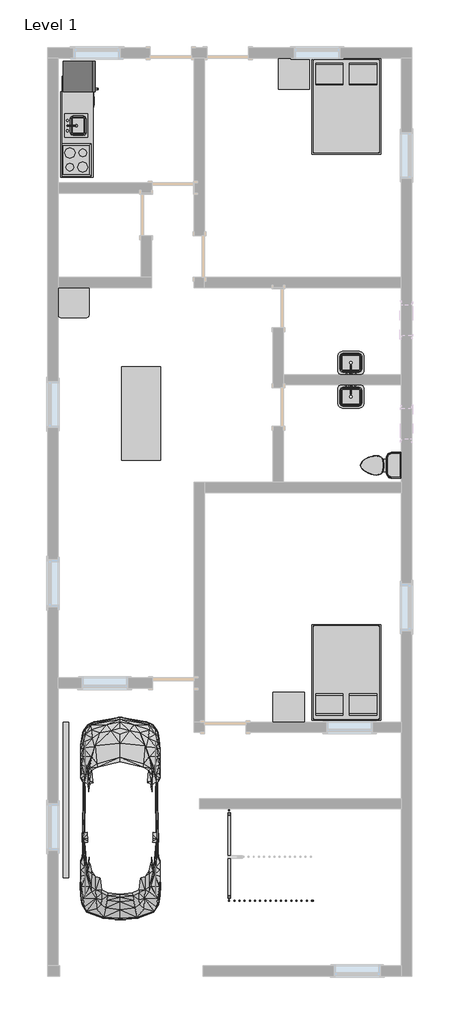
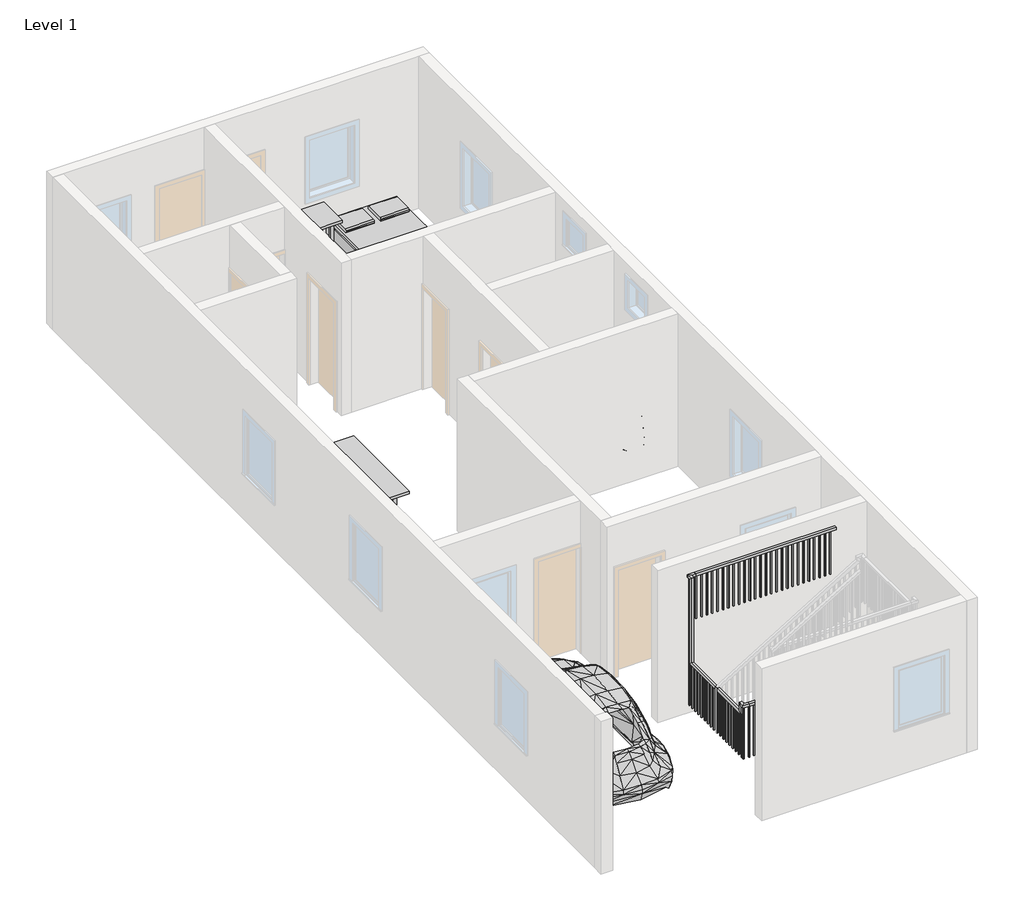
# One storey, part 3 of 3: 7 furniture elements, 6 proxies, 4 flow terminals, 1 railing.
"""IFC4 building model written with IfcOpenShell, lengths in millimetres."""

from ifc_helpers import new_model, si_unit, frame, origin, place, context, project, spatial, polyline, outline, extrude, faceted_brep, transform, mapped, element, save
from components import proxy_a6faaae8, proxy_45b28599, kitchenette_medium_kitchenette_medium_844211aa, parking_space_9_x_18_90_deg_2dcab977, rpc_beetle_rpc_beetle_3ce7ba48, proxy_c523a7b7, flow_terminal_871c2e40, flow_terminal_62a433f7, toilet_domestic_3d_toilet_domestic_3d_f7549cf7, toilet_domestic_3d_toilet_domestic_3d_183bbd19, furniture_c8abb964, furniture_1781b5df, furniture_bcf351fa, furniture_5bc9ed15, furniture_a5b052b6

model = new_model("IFC4")

# Units and contexts
model_context = context("Model", 3, world=origin())
ifc_project = project(units=[si_unit("LENGTHUNIT", "METRE", prefix="MILLI")], contexts=[model_context])

# Site, building, storey
site = spatial("IfcSite", under=ifc_project)
building = spatial("IfcBuilding", under=site)
storey = spatial("IfcBuildingStorey", under=building, Name="Level 1", Elevation=0.0)

# Proxies
placement = place(None, origin())
proxy_shape = proxy_a6faaae8(model_context)
element("IfcBuildingElementProxy", 1, Name="Cook Top-4 Unit2 : 22\" x 20\"", ObjectType="Cook Top-4 Unit2 : 22\" x 20\"", at=placement, inside=storey, context=model_context, shape_type="MappedRepresentation", body=[
    mapped(proxy_shape, transform((-9361.8283387, 8629.5865244, 0.0), x_axis=(0.0, 1.0, 0.0), y_axis=(-1.0, 0.0, 0.0), z_axis=(0.0, 0.0, 1.0))),
])
proxy_2_shape = proxy_45b28599(model_context)
element("IfcBuildingElementProxy", 2, Name="Dishwasher : 24\" x 24\" x 34\"", ObjectType="Dishwasher : 24\" x 24\" x 34\"", at=placement, inside=storey, context=model_context, shape_type="MappedRepresentation", body=[
    mapped(proxy_2_shape, transform((-9069.978774, 9580.7690559, 0.0), x_axis=(0.0, 1.0, 0.0), y_axis=(-1.0, 0.0, 0.0), z_axis=(0.0, 0.0, 1.0))),
])
kitchenette_medium_kitchenette_medium_shape = kitchenette_medium_kitchenette_medium_844211aa(model_context)
element("IfcBuildingElementProxy", 3, Name="Kitchenette - Medium : Kitchenette - Medium", ObjectType="Kitchenette - Medium : Kitchenette - Medium", at=placement, inside=storey, context=model_context, shape_type="MappedRepresentation", body=[
    mapped(kitchenette_medium_kitchenette_medium_shape, transform((-9666.6283387, 8953.7488195, 0.0), x_axis=(0.0, 1.0, 0.0), y_axis=(-1.0, 0.0, 0.0), z_axis=(0.0, 0.0, 1.0))),
])
parking_space_9_x_18_90_deg_shape = parking_space_9_x_18_90_deg_2dcab977(model_context)
element("IfcBuildingElementProxy", 4, Name="Parking Space : 9' x 18' - 90 deg", ObjectType="Parking Space : 9' x 18' - 90 deg", at=placement, inside=storey, context=model_context, shape_type="MappedRepresentation", body=[
    mapped(parking_space_9_x_18_90_deg_shape, transform((-9564.1370113, -2381.3134756, 0.0), x_axis=(1.0, 0.0, 0.0), y_axis=(0.0, 1.0, 0.0), z_axis=(0.0, 0.0, 1.0))),
])
rpc_beetle_rpc_beetle_shape = rpc_beetle_rpc_beetle_3ce7ba48(model_context)
element("IfcBuildingElementProxy", 5, Name="RPC Beetle : RPC Beetle", ObjectType="RPC Beetle : RPC Beetle", at=placement, inside=storey, context=model_context, shape_type="MappedRepresentation", body=[
    mapped(rpc_beetle_rpc_beetle_shape, transform((-8497.3370113, -5505.5134756, 0.0), x_axis=(1.0, 0.0, 0.0), y_axis=(0.0, 1.0, 0.0), z_axis=(0.0, 0.0, 1.0))),
])
proxy_3_shape = proxy_c523a7b7(model_context)
element("IfcBuildingElementProxy", 6, Name="Refrigerator : 24\" x 25\" LH", ObjectType="Refrigerator : 24\" x 25\" LH", at=placement, inside=storey, context=model_context, shape_type="MappedRepresentation", body=[
    mapped(proxy_3_shape, transform((-9316.1793673, 10261.5365244, 0.0), x_axis=(0.0, 1.0, 0.0), y_axis=(-1.0, 0.0, 0.0), z_axis=(0.0, 0.0, 1.0))),
])

# Flow terminals
flow_terminal_shape = flow_terminal_871c2e40(model_context)
element("IfcFlowTerminal", 7, ObjectType="Sink Kitchen-Island : 18\" x 18\"", at=placement, inside=storey, context=model_context, shape_type="MappedRepresentation", body=[
    mapped(flow_terminal_shape, transform((-9359.4829376, 9286.9972838, -14.4), x_axis=(0.0, 1.0, 0.0), y_axis=(-1.0, 0.0, 0.0), z_axis=(0.0, 0.0, 1.0))),
])
flow_terminal_2_shape = flow_terminal_62a433f7(model_context)
element("IfcFlowTerminal", 8, ObjectType="Sink Vanity-Square : 20\" x 18\"", at=placement, inside=storey, context=model_context, shape_type="MappedRepresentation", body=[
    mapped(flow_terminal_2_shape, transform((-3960.4477707, 4606.0319255, 0.0), x_axis=(-1.0000000000000004, 0.0, 0.0), y_axis=(0.0, -1.0000000000000004, 0.0), z_axis=(0.0, 0.0, 1.0))),
])
element("IfcFlowTerminal", 9, ObjectType="Sink Vanity-Square : 20\" x 18\"", at=placement, inside=storey, context=model_context, shape_type="MappedRepresentation", body=[
    mapped(flow_terminal_2_shape, transform((-3991.8262519, 4042.5411233, 0.0), x_axis=(1.0, 0.0, 0.0), y_axis=(0.0, 1.0, 0.0), z_axis=(0.0, 0.0, 1.0))),
])
toilet_domestic_3d_toilet_domestic_3d_shape = toilet_domestic_3d_toilet_domestic_3d_f7549cf7(model_context)
toilet_domestic_3d_toilet_domestic_3d_2_shape = toilet_domestic_3d_toilet_domestic_3d_183bbd19(model_context)
element("IfcFlowTerminal", 10, ObjectType="Toilet-Domestic-3D : Toilet-Domestic-3D", at=placement, inside=storey, context=model_context, shape_type="MappedRepresentation", body=[
    mapped(toilet_domestic_3d_toilet_domestic_3d_shape, transform((-3480.2330387, 2647.8865244, 0.0), x_axis=(0.0, -1.0000000000000004, 0.0), y_axis=(1.0000000000000004, 0.0, 0.0), z_axis=(0.0, 0.0, 1.0))),
    mapped(toilet_domestic_3d_toilet_domestic_3d_2_shape, transform((-3480.2330387, 2647.8865244, 0.0), x_axis=(0.0, -1.0000000000000004, 0.0), y_axis=(1.0000000000000004, 0.0, 0.0), z_axis=(0.0, 0.0, 1.0))),
])

# Furniture
furniture_shape = furniture_c8abb964(model_context)
element("IfcFurniture", 11, ObjectType="Bed-Box : Double 53\" x 74\"", at=placement, inside=storey, context=model_context, shape_type="MappedRepresentation", body=[
    mapped(furniture_shape, transform((-4404.1894703, 9918.1160326, 0.0), x_axis=(1.0, 0.0, 0.0), y_axis=(0.0, 1.0, 0.0), z_axis=(0.0, 0.0, 1.0))),
])
element("IfcFurniture", 12, ObjectType="Bed-Box : Double 53\" x 74\"", at=placement, inside=storey, context=model_context, shape_type="MappedRepresentation", body=[
    mapped(furniture_shape, transform((-3725.8845523, -1644.7134756, 0.0), x_axis=(-1.0000000000000004, 0.0, 0.0), y_axis=(0.0, -1.0000000000000004, 0.0), z_axis=(0.0, 0.0, 1.0))),
])
furniture_2_shape = furniture_1781b5df(model_context)
element("IfcFurniture", 13, ObjectType="Counter Top w Sink Hole : 24\" Depth", at=placement, inside=storey, context=model_context, shape_type="MappedRepresentation", body=[
    mapped(furniture_2_shape, transform((-9666.6283387, 9487.1488195, -14.4), x_axis=(0.0, 1.0, 0.0), y_axis=(-1.0, 0.0, 0.0), z_axis=(0.0, 0.0, 1.0))),
])
furniture_3_shape = furniture_bcf351fa(model_context)
element("IfcFurniture", 14, ObjectType="Table-End : 24\" x 24\"", at=placement, inside=storey, context=model_context, shape_type="MappedRepresentation", body=[
    mapped(furniture_3_shape, transform((-9720.2706416, 5695.8865244, 0.0), x_axis=(1.0, 0.0, 0.0), y_axis=(0.0, 1.0, 0.0), z_axis=(0.0, 0.0, 1.0))),
])
furniture_4_shape = furniture_5bc9ed15(model_context)
element("IfcFurniture", 15, ObjectType="Table-Night Stand : 24\" x 24\" x 30\"", at=placement, inside=storey, context=model_context, shape_type="MappedRepresentation", body=[
    mapped(furniture_4_shape, transform((-5503.8706416, -2406.7134756, 0.0), x_axis=(1.0, 0.0, 0.0), y_axis=(0.0, 1.0, 0.0), z_axis=(0.0, 0.0, 1.0))),
])
element("IfcFurniture", 16, ObjectType="Table-Night Stand : 24\" x 24\" x 30\"", at=placement, inside=storey, context=model_context, shape_type="MappedRepresentation", body=[
    mapped(furniture_4_shape, transform((-5402.2706416, 10013.8865244, 0.0), x_axis=(1.0, 0.0, 0.0), y_axis=(0.0, 1.0, 0.0), z_axis=(0.0, 0.0, 1.0))),
])
furniture_5_shape = furniture_a5b052b6(model_context)
element("IfcFurniture", 17, ObjectType="Table-Rectangular : 72\" x 30\"", at=placement, inside=storey, context=model_context, shape_type="MappedRepresentation", body=[
    mapped(furniture_5_shape, transform((-8090.9370113, 3663.8865244, 0.0), x_axis=(0.0, 1.0, 0.0), y_axis=(-1.0, 0.0, 0.0), z_axis=(0.0, 0.0, 1.0))),
])

# Railing
element("IfcRailing", 18, ObjectType="Handrail - Rectangular", at=placement, inside=storey, context=model_context, shape_type="SolidModel", body=[
    faceted_brep([(-4712.7370113, -5909.6215145, 1253.0666667), (-4712.7370113, -5909.6215145, 1202.2666667), (-4712.7370113, -5858.8215145, 1202.2666667), (-4712.7370113, -5858.8215145, 1253.0666667), (-6262.1370113, -5909.6215145, 1253.0666667), (-6262.1370113, -5909.6215145, 1202.2666667), (-6262.1370113, -5858.8215145, 1202.2666667), (-6262.1370113, -5858.8215145, 1253.0666667), (-6389.1370113, -5909.6215145, 1253.0666667), (-6389.1370113, -5909.6215145, 1202.2666667), (-6338.3370113, -5858.8215145, 1202.2666667), (-6338.3370113, -5858.8215145, 1253.0666667), (-6389.1370113, -5782.6215145, 1253.0666667), (-6389.1370113, -5833.4215145, 1202.2666667), (-6338.3370113, -5833.4215145, 1202.2666667), (-6338.3370113, -5782.6215145, 1253.0666667), (-6389.1370113, -5782.6215145, 1083.7333333), (-6389.1370113, -5833.4215145, 1032.9333333), (-6338.3370113, -5833.4215145, 1032.9333333), (-6338.3370113, -5782.6215145, 1083.7333333), (-6389.1370113, -4211.9518521, 1083.7333333), (-6389.1370113, -4161.1518521, 1032.9333333), (-6338.3370113, -4161.1518521, 1032.9333333), (-6338.3370113, -4211.9518521, 1083.7333333), (-6389.1370113, -4211.9518521, 2777.0666667), (-6389.1370113, -4161.1518521, 2726.2666667), (-6338.3370113, -4161.1518521, 2726.2666667), (-6338.3370113, -4211.9518521, 2777.0666667), (-6389.1370113, -4084.9518521, 2777.0666667), (-6389.1370113, -4084.9518521, 2726.2666667), (-6338.3370113, -4135.7518521, 2726.2666667), (-6338.3370113, -4135.7518521, 2777.0666667), (-6262.1370113, -4084.9518521, 2777.0666667), (-6262.1370113, -4084.9518521, 2726.2666667), (-6262.1370113, -4135.7518521, 2726.2666667), (-6262.1370113, -4135.7518521, 2777.0666667), (-3595.1370113, -4084.9518521, 2777.0666667), (-3595.1370113, -4135.7518521, 2777.0666667), (-3595.1370113, -4135.7518521, 2726.2666667), (-3595.1370113, -4084.9518521, 2726.2666667)], [[[0, 1, 2, 3]], [[1, 0, 4, 5]], [[2, 1, 5, 6]], [[3, 2, 6, 7]], [[0, 3, 7, 4]], [[5, 4, 8, 9]], [[6, 5, 9, 10]], [[7, 6, 10, 11]], [[4, 7, 11, 8]], [[9, 8, 12, 13]], [[10, 9, 13, 14]], [[11, 10, 14, 15]], [[8, 11, 15, 12]], [[13, 12, 16, 17]], [[14, 13, 17, 18]], [[15, 14, 18, 19]], [[12, 15, 19, 16]], [[17, 16, 20, 21]], [[18, 17, 21, 22]], [[19, 18, 22, 23]], [[16, 19, 23, 20]], [[21, 20, 24, 25]], [[22, 21, 25, 26]], [[23, 22, 26, 27]], [[20, 23, 27, 24]], [[25, 24, 28, 29]], [[26, 25, 29, 30]], [[27, 26, 30, 31]], [[24, 27, 31, 28]], [[29, 28, 32, 33]], [[30, 29, 33, 34]], [[31, 30, 34, 35]], [[28, 31, 35, 32]], [[36, 37, 38, 39]], [[33, 32, 36, 39]], [[34, 33, 39, 38]], [[35, 34, 38, 37]], [[32, 35, 37, 36]]]),
    faceted_brep([(-3595.1370113, -4084.9518521, 2777.0666667), (-3595.1370113, -4084.9518521, 2726.2666667), (-3595.1370113, -4034.1518521, 2726.2666667), (-3595.1370113, -4034.1518521, 2777.0666667), (-6389.1370113, -4084.9518521, 2777.0666667), (-6389.1370113, -4034.1518521, 2777.0666667), (-6389.1370113, -4034.1518521, 2726.2666667), (-6389.1370113, -4084.9518521, 2726.2666667)], [[[0, 1, 2, 3]], [[4, 5, 6, 7]], [[1, 0, 4, 7]], [[2, 1, 7, 6]], [[3, 2, 6, 5]], [[0, 3, 5, 4]]]),
    extrude(outline(polyline([(-4747.6620113, -5893.7465145), (-4747.6620113, -5874.6965145), (-4728.6120113, -5874.6965145), (-4728.6120113, -5893.7465145), (-4747.6620113, -5893.7465145)])), frame((0.0, 0.0, 169.3333333), z_axis=(0.0, 0.0, 1.0), x_axis=(1.0, 0.0, 0.0)), (0.0, 0.0, 1.0), 1032.9333333),
    extrude(outline(polyline([(-4849.2620113, -5893.7465145), (-4849.2620113, -5874.6965145), (-4830.2120113, -5874.6965145), (-4830.2120113, -5893.7465145), (-4849.2620113, -5893.7465145)])), frame((0.0, 0.0, 169.3333333), z_axis=(0.0, 0.0, 1.0), x_axis=(1.0, 0.0, 0.0)), (0.0, 0.0, 1.0), 1032.9333333),
    extrude(outline(polyline([(-4950.8620113, -5893.7465145), (-4950.8620113, -5874.6965145), (-4931.8120113, -5874.6965145), (-4931.8120113, -5893.7465145), (-4950.8620113, -5893.7465145)])), frame((0.0, 0.0, 169.3333333), z_axis=(0.0, 0.0, 1.0), x_axis=(1.0, 0.0, 0.0)), (0.0, 0.0, 1.0), 1032.9333333),
    extrude(outline(polyline([(-5052.4620113, -5893.7465145), (-5052.4620113, -5874.6965145), (-5033.4120113, -5874.6965145), (-5033.4120113, -5893.7465145), (-5052.4620113, -5893.7465145)])), frame((0.0, 0.0, 169.3333333), z_axis=(0.0, 0.0, 1.0), x_axis=(1.0, 0.0, 0.0)), (0.0, 0.0, 1.0), 1032.9333333),
    extrude(outline(polyline([(-5154.0620113, -5893.7465145), (-5154.0620113, -5874.6965145), (-5135.0120113, -5874.6965145), (-5135.0120113, -5893.7465145), (-5154.0620113, -5893.7465145)])), frame((0.0, 0.0, 169.3333333), z_axis=(0.0, 0.0, 1.0), x_axis=(1.0, 0.0, 0.0)), (0.0, 0.0, 1.0), 1032.9333333),
    extrude(outline(polyline([(-5255.6620113, -5893.7465145), (-5255.6620113, -5874.6965145), (-5236.6120113, -5874.6965145), (-5236.6120113, -5893.7465145), (-5255.6620113, -5893.7465145)])), frame((0.0, 0.0, 169.3333333), z_axis=(0.0, 0.0, 1.0), x_axis=(1.0, 0.0, 0.0)), (0.0, 0.0, 1.0), 1032.9333333),
    extrude(outline(polyline([(-5357.2620113, -5893.7465145), (-5357.2620113, -5874.6965145), (-5338.2120113, -5874.6965145), (-5338.2120113, -5893.7465145), (-5357.2620113, -5893.7465145)])), frame((0.0, 0.0, 169.3333333), z_axis=(0.0, 0.0, 1.0), x_axis=(1.0, 0.0, 0.0)), (0.0, 0.0, 1.0), 1032.9333333),
    extrude(outline(polyline([(-5458.8620113, -5893.7465145), (-5458.8620113, -5874.6965145), (-5439.8120113, -5874.6965145), (-5439.8120113, -5893.7465145), (-5458.8620113, -5893.7465145)])), frame((0.0, 0.0, 169.3333333), z_axis=(0.0, 0.0, 1.0), x_axis=(1.0, 0.0, 0.0)), (0.0, 0.0, 1.0), 1032.9333333),
    extrude(outline(polyline([(-5560.4620113, -5893.7465145), (-5560.4620113, -5874.6965145), (-5541.4120113, -5874.6965145), (-5541.4120113, -5893.7465145), (-5560.4620113, -5893.7465145)])), frame((0.0, 0.0, 169.3333333), z_axis=(0.0, 0.0, 1.0), x_axis=(1.0, 0.0, 0.0)), (0.0, 0.0, 1.0), 1032.9333333),
    extrude(outline(polyline([(-5662.0620113, -5893.7465145), (-5662.0620113, -5874.6965145), (-5643.0120113, -5874.6965145), (-5643.0120113, -5893.7465145), (-5662.0620113, -5893.7465145)])), frame((0.0, 0.0, 169.3333333), z_axis=(0.0, 0.0, 1.0), x_axis=(1.0, 0.0, 0.0)), (0.0, 0.0, 1.0), 1032.9333333),
    extrude(outline(polyline([(-5763.6620113, -5893.7465145), (-5763.6620113, -5874.6965145), (-5744.6120113, -5874.6965145), (-5744.6120113, -5893.7465145), (-5763.6620113, -5893.7465145)])), frame((0.0, 0.0, 169.3333333), z_axis=(0.0, 0.0, 1.0), x_axis=(1.0, 0.0, 0.0)), (0.0, 0.0, 1.0), 1032.9333333),
    extrude(outline(polyline([(-5865.2620113, -5893.7465145), (-5865.2620113, -5874.6965145), (-5846.2120113, -5874.6965145), (-5846.2120113, -5893.7465145), (-5865.2620113, -5893.7465145)])), frame((0.0, 0.0, 169.3333333), z_axis=(0.0, 0.0, 1.0), x_axis=(1.0, 0.0, 0.0)), (0.0, 0.0, 1.0), 1032.9333333),
    extrude(outline(polyline([(-5966.8620113, -5893.7465145), (-5966.8620113, -5874.6965145), (-5947.8120113, -5874.6965145), (-5947.8120113, -5893.7465145), (-5966.8620113, -5893.7465145)])), frame((0.0, 0.0, 169.3333333), z_axis=(0.0, 0.0, 1.0), x_axis=(1.0, 0.0, 0.0)), (0.0, 0.0, 1.0), 1032.9333333),
    extrude(outline(polyline([(-6068.4620113, -5893.7465145), (-6068.4620113, -5874.6965145), (-6049.4120113, -5874.6965145), (-6049.4120113, -5893.7465145), (-6068.4620113, -5893.7465145)])), frame((0.0, 0.0, 169.3333333), z_axis=(0.0, 0.0, 1.0), x_axis=(1.0, 0.0, 0.0)), (0.0, 0.0, 1.0), 1032.9333333),
    extrude(outline(polyline([(-6170.0620113, -5893.7465145), (-6170.0620113, -5874.6965145), (-6151.0120113, -5874.6965145), (-6151.0120113, -5893.7465145), (-6170.0620113, -5893.7465145)])), frame((0.0, 0.0, 169.3333333), z_axis=(0.0, 0.0, 1.0), x_axis=(1.0, 0.0, 0.0)), (0.0, 0.0, 1.0), 1032.9333333),
    extrude(outline(polyline([(-6271.6620113, -5893.7465145), (-6271.6620113, -5874.6965145), (-6252.6120113, -5874.6965145), (-6252.6120113, -5893.7465145), (-6271.6620113, -5893.7465145)])), frame((0.0, 0.0, 169.3333333), z_axis=(0.0, 0.0, 1.0), x_axis=(1.0, 0.0, 0.0)), (0.0, 0.0, 1.0), 1032.9333333),
    extrude(outline(polyline([(-6373.2620113, -5828.0268521), (-6354.2120113, -5828.0268521), (-6354.2120113, -5847.0768521), (-6373.2620113, -5847.0768521), (-6373.2620113, -5828.0268521)])), frame((0.0, 0.0, 169.3333333), z_axis=(0.0, 0.0, 1.0), x_axis=(1.0, 0.0, 0.0)), (0.0, 0.0, 1.0), 863.6),
    extrude(outline(polyline([(-6373.2620113, -5726.4268521), (-6354.2120113, -5726.4268521), (-6354.2120113, -5745.4768521), (-6373.2620113, -5745.4768521), (-6373.2620113, -5726.4268521)])), frame((0.0, 0.0, 169.3333333), z_axis=(0.0, 0.0, 1.0), x_axis=(1.0, 0.0, 0.0)), (0.0, 0.0, 1.0), 863.6),
    extrude(outline(polyline([(-6373.2620113, -5624.8268521), (-6354.2120113, -5624.8268521), (-6354.2120113, -5643.8768521), (-6373.2620113, -5643.8768521), (-6373.2620113, -5624.8268521)])), frame((0.0, 0.0, 169.3333333), z_axis=(0.0, 0.0, 1.0), x_axis=(1.0, 0.0, 0.0)), (0.0, 0.0, 1.0), 863.6),
    extrude(outline(polyline([(-6373.2620113, -5523.2268521), (-6354.2120113, -5523.2268521), (-6354.2120113, -5542.2768521), (-6373.2620113, -5542.2768521), (-6373.2620113, -5523.2268521)])), frame((0.0, 0.0, 169.3333333), z_axis=(0.0, 0.0, 1.0), x_axis=(1.0, 0.0, 0.0)), (0.0, 0.0, 1.0), 863.6),
    extrude(outline(polyline([(-6373.2620113, -5421.6268521), (-6354.2120113, -5421.6268521), (-6354.2120113, -5440.6768521), (-6373.2620113, -5440.6768521), (-6373.2620113, -5421.6268521)])), frame((0.0, 0.0, 169.3333333), z_axis=(0.0, 0.0, 1.0), x_axis=(1.0, 0.0, 0.0)), (0.0, 0.0, 1.0), 863.6),
    extrude(outline(polyline([(-6373.2620113, -5320.0268521), (-6354.2120113, -5320.0268521), (-6354.2120113, -5339.0768521), (-6373.2620113, -5339.0768521), (-6373.2620113, -5320.0268521)])), frame((0.0, 0.0, 169.3333333), z_axis=(0.0, 0.0, 1.0), x_axis=(1.0, 0.0, 0.0)), (0.0, 0.0, 1.0), 863.6),
    extrude(outline(polyline([(-6373.2620113, -5218.4268521), (-6354.2120113, -5218.4268521), (-6354.2120113, -5237.4768521), (-6373.2620113, -5237.4768521), (-6373.2620113, -5218.4268521)])), frame((0.0, 0.0, 169.3333333), z_axis=(0.0, 0.0, 1.0), x_axis=(1.0, 0.0, 0.0)), (0.0, 0.0, 1.0), 863.6),
    extrude(outline(polyline([(-6373.2620113, -5116.8268521), (-6354.2120113, -5116.8268521), (-6354.2120113, -5135.8768521), (-6373.2620113, -5135.8768521), (-6373.2620113, -5116.8268521)])), frame((0.0, 0.0, 169.3333333), z_axis=(0.0, 0.0, 1.0), x_axis=(1.0, 0.0, 0.0)), (0.0, 0.0, 1.0), 863.6),
    extrude(outline(polyline([(-6373.2620113, -5015.2268521), (-6354.2120113, -5015.2268521), (-6354.2120113, -5034.2768521), (-6373.2620113, -5034.2768521), (-6373.2620113, -5015.2268521)])), frame((0.0, 0.0, 169.3333333), z_axis=(0.0, 0.0, 1.0), x_axis=(1.0, 0.0, 0.0)), (0.0, 0.0, 1.0), 863.6),
    extrude(outline(polyline([(-6373.2620113, -4913.6268521), (-6354.2120113, -4913.6268521), (-6354.2120113, -4932.6768521), (-6373.2620113, -4932.6768521), (-6373.2620113, -4913.6268521)])), frame((0.0, 0.0, 169.3333333), z_axis=(0.0, 0.0, 1.0), x_axis=(1.0, 0.0, 0.0)), (0.0, 0.0, 1.0), 863.6),
    extrude(outline(polyline([(-6373.2620113, -4812.0268521), (-6354.2120113, -4812.0268521), (-6354.2120113, -4831.0768521), (-6373.2620113, -4831.0768521), (-6373.2620113, -4812.0268521)])), frame((0.0, 0.0, 169.3333333), z_axis=(0.0, 0.0, 1.0), x_axis=(1.0, 0.0, 0.0)), (0.0, 0.0, 1.0), 863.6),
    extrude(outline(polyline([(-6373.2620113, -4710.4268521), (-6354.2120113, -4710.4268521), (-6354.2120113, -4729.4768521), (-6373.2620113, -4729.4768521), (-6373.2620113, -4710.4268521)])), frame((0.0, 0.0, 169.3333333), z_axis=(0.0, 0.0, 1.0), x_axis=(1.0, 0.0, 0.0)), (0.0, 0.0, 1.0), 863.6),
    extrude(outline(polyline([(-6373.2620113, -4608.8268521), (-6354.2120113, -4608.8268521), (-6354.2120113, -4627.8768521), (-6373.2620113, -4627.8768521), (-6373.2620113, -4608.8268521)])), frame((0.0, 0.0, 169.3333333), z_axis=(0.0, 0.0, 1.0), x_axis=(1.0, 0.0, 0.0)), (0.0, 0.0, 1.0), 863.6),
    extrude(outline(polyline([(-6373.2620113, -4507.2268521), (-6354.2120113, -4507.2268521), (-6354.2120113, -4526.2768521), (-6373.2620113, -4526.2768521), (-6373.2620113, -4507.2268521)])), frame((0.0, 0.0, 169.3333333), z_axis=(0.0, 0.0, 1.0), x_axis=(1.0, 0.0, 0.0)), (0.0, 0.0, 1.0), 863.6),
    extrude(outline(polyline([(-6373.2620113, -4405.6268521), (-6354.2120113, -4405.6268521), (-6354.2120113, -4424.6768521), (-6373.2620113, -4424.6768521), (-6373.2620113, -4405.6268521)])), frame((0.0, 0.0, 169.3333333), z_axis=(0.0, 0.0, 1.0), x_axis=(1.0, 0.0, 0.0)), (0.0, 0.0, 1.0), 863.6),
    extrude(outline(polyline([(-6373.2620113, -4304.0268521), (-6354.2120113, -4304.0268521), (-6354.2120113, -4323.0768521), (-6373.2620113, -4323.0768521), (-6373.2620113, -4304.0268521)])), frame((0.0, 0.0, 169.3333333), z_axis=(0.0, 0.0, 1.0), x_axis=(1.0, 0.0, 0.0)), (0.0, 0.0, 1.0), 863.6),
    extrude(outline(polyline([(-6373.2620113, -4202.4268521), (-6354.2120113, -4202.4268521), (-6354.2120113, -4221.4768521), (-6373.2620113, -4221.4768521), (-6373.2620113, -4202.4268521)])), frame((0.0, 0.0, 169.3333333), z_axis=(0.0, 0.0, 1.0), x_axis=(1.0, 0.0, 0.0)), (0.0, 0.0, 1.0), 863.6),
    extrude(outline(polyline([(-6328.8120113, -4100.8268521), (-6328.8120113, -4119.8768521), (-6347.8620113, -4119.8768521), (-6347.8620113, -4100.8268521), (-6328.8120113, -4100.8268521)])), frame((0.0, 0.0, 1862.6666667), z_axis=(0.0, 0.0, 1.0), x_axis=(1.0, 0.0, 0.0)), (0.0, 0.0, 1.0), 863.6),
    extrude(outline(polyline([(-6227.2120113, -4100.8268521), (-6227.2120113, -4119.8768521), (-6246.2620113, -4119.8768521), (-6246.2620113, -4100.8268521), (-6227.2120113, -4100.8268521)])), frame((0.0, 0.0, 1862.6666667), z_axis=(0.0, 0.0, 1.0), x_axis=(1.0, 0.0, 0.0)), (0.0, 0.0, 1.0), 863.6),
    extrude(outline(polyline([(-6125.6120113, -4100.8268521), (-6125.6120113, -4119.8768521), (-6144.6620113, -4119.8768521), (-6144.6620113, -4100.8268521), (-6125.6120113, -4100.8268521)])), frame((0.0, 0.0, 1862.6666667), z_axis=(0.0, 0.0, 1.0), x_axis=(1.0, 0.0, 0.0)), (0.0, 0.0, 1.0), 863.6),
    extrude(outline(polyline([(-6024.0120113, -4100.8268521), (-6024.0120113, -4119.8768521), (-6043.0620113, -4119.8768521), (-6043.0620113, -4100.8268521), (-6024.0120113, -4100.8268521)])), frame((0.0, 0.0, 1862.6666667), z_axis=(0.0, 0.0, 1.0), x_axis=(1.0, 0.0, 0.0)), (0.0, 0.0, 1.0), 863.6),
    extrude(outline(polyline([(-5922.4120113, -4100.8268521), (-5922.4120113, -4119.8768521), (-5941.4620113, -4119.8768521), (-5941.4620113, -4100.8268521), (-5922.4120113, -4100.8268521)])), frame((0.0, 0.0, 1862.6666667), z_axis=(0.0, 0.0, 1.0), x_axis=(1.0, 0.0, 0.0)), (0.0, 0.0, 1.0), 863.6),
    extrude(outline(polyline([(-5820.8120113, -4100.8268521), (-5820.8120113, -4119.8768521), (-5839.8620113, -4119.8768521), (-5839.8620113, -4100.8268521), (-5820.8120113, -4100.8268521)])), frame((0.0, 0.0, 1862.6666667), z_axis=(0.0, 0.0, 1.0), x_axis=(1.0, 0.0, 0.0)), (0.0, 0.0, 1.0), 863.6),
    extrude(outline(polyline([(-5719.2120113, -4100.8268521), (-5719.2120113, -4119.8768521), (-5738.2620113, -4119.8768521), (-5738.2620113, -4100.8268521), (-5719.2120113, -4100.8268521)])), frame((0.0, 0.0, 1862.6666667), z_axis=(0.0, 0.0, 1.0), x_axis=(1.0, 0.0, 0.0)), (0.0, 0.0, 1.0), 863.6),
    extrude(outline(polyline([(-5617.6120113, -4100.8268521), (-5617.6120113, -4119.8768521), (-5636.6620113, -4119.8768521), (-5636.6620113, -4100.8268521), (-5617.6120113, -4100.8268521)])), frame((0.0, 0.0, 1862.6666667), z_axis=(0.0, 0.0, 1.0), x_axis=(1.0, 0.0, 0.0)), (0.0, 0.0, 1.0), 863.6),
    extrude(outline(polyline([(-5516.0120113, -4100.8268521), (-5516.0120113, -4119.8768521), (-5535.0620113, -4119.8768521), (-5535.0620113, -4100.8268521), (-5516.0120113, -4100.8268521)])), frame((0.0, 0.0, 1862.6666667), z_axis=(0.0, 0.0, 1.0), x_axis=(1.0, 0.0, 0.0)), (0.0, 0.0, 1.0), 863.6),
    extrude(outline(polyline([(-5414.4120113, -4100.8268521), (-5414.4120113, -4119.8768521), (-5433.4620113, -4119.8768521), (-5433.4620113, -4100.8268521), (-5414.4120113, -4100.8268521)])), frame((0.0, 0.0, 1862.6666667), z_axis=(0.0, 0.0, 1.0), x_axis=(1.0, 0.0, 0.0)), (0.0, 0.0, 1.0), 863.6),
    extrude(outline(polyline([(-5312.8120113, -4100.8268521), (-5312.8120113, -4119.8768521), (-5331.8620113, -4119.8768521), (-5331.8620113, -4100.8268521), (-5312.8120113, -4100.8268521)])), frame((0.0, 0.0, 1862.6666667), z_axis=(0.0, 0.0, 1.0), x_axis=(1.0, 0.0, 0.0)), (0.0, 0.0, 1.0), 863.6),
    extrude(outline(polyline([(-5211.2120113, -4100.8268521), (-5211.2120113, -4119.8768521), (-5230.2620113, -4119.8768521), (-5230.2620113, -4100.8268521), (-5211.2120113, -4100.8268521)])), frame((0.0, 0.0, 1862.6666667), z_axis=(0.0, 0.0, 1.0), x_axis=(1.0, 0.0, 0.0)), (0.0, 0.0, 1.0), 863.6),
    extrude(outline(polyline([(-5109.6120113, -4100.8268521), (-5109.6120113, -4119.8768521), (-5128.6620113, -4119.8768521), (-5128.6620113, -4100.8268521), (-5109.6120113, -4100.8268521)])), frame((0.0, 0.0, 1862.6666667), z_axis=(0.0, 0.0, 1.0), x_axis=(1.0, 0.0, 0.0)), (0.0, 0.0, 1.0), 863.6),
    extrude(outline(polyline([(-5008.0120113, -4100.8268521), (-5008.0120113, -4119.8768521), (-5027.0620113, -4119.8768521), (-5027.0620113, -4100.8268521), (-5008.0120113, -4100.8268521)])), frame((0.0, 0.0, 1862.6666667), z_axis=(0.0, 0.0, 1.0), x_axis=(1.0, 0.0, 0.0)), (0.0, 0.0, 1.0), 863.6),
    extrude(outline(polyline([(-4906.4120113, -4100.8268521), (-4906.4120113, -4119.8768521), (-4925.4620113, -4119.8768521), (-4925.4620113, -4100.8268521), (-4906.4120113, -4100.8268521)])), frame((0.0, 0.0, 1862.6666667), z_axis=(0.0, 0.0, 1.0), x_axis=(1.0, 0.0, 0.0)), (0.0, 0.0, 1.0), 863.6),
    extrude(outline(polyline([(-4804.8120113, -4100.8268521), (-4804.8120113, -4119.8768521), (-4823.8620113, -4119.8768521), (-4823.8620113, -4100.8268521), (-4804.8120113, -4100.8268521)])), frame((0.0, 0.0, 1862.6666667), z_axis=(0.0, 0.0, 1.0), x_axis=(1.0, 0.0, 0.0)), (0.0, 0.0, 1.0), 863.6),
    extrude(outline(polyline([(-4703.2120113, -4100.8268521), (-4703.2120113, -4119.8768521), (-4722.2620113, -4119.8768521), (-4722.2620113, -4100.8268521), (-4703.2120113, -4100.8268521)])), frame((0.0, 0.0, 1862.6666667), z_axis=(0.0, 0.0, 1.0), x_axis=(1.0, 0.0, 0.0)), (0.0, 0.0, 1.0), 863.6),
    extrude(outline(polyline([(-4601.6120113, -4100.8268521), (-4601.6120113, -4119.8768521), (-4620.6620113, -4119.8768521), (-4620.6620113, -4100.8268521), (-4601.6120113, -4100.8268521)])), frame((0.0, 0.0, 1862.6666667), z_axis=(0.0, 0.0, 1.0), x_axis=(1.0, 0.0, 0.0)), (0.0, 0.0, 1.0), 863.6),
    extrude(outline(polyline([(-4500.0120113, -4100.8268521), (-4500.0120113, -4119.8768521), (-4519.0620113, -4119.8768521), (-4519.0620113, -4100.8268521), (-4500.0120113, -4100.8268521)])), frame((0.0, 0.0, 1862.6666667), z_axis=(0.0, 0.0, 1.0), x_axis=(1.0, 0.0, 0.0)), (0.0, 0.0, 1.0), 863.6),
    extrude(outline(polyline([(-4398.4120113, -4100.8268521), (-4398.4120113, -4119.8768521), (-4417.4620113, -4119.8768521), (-4417.4620113, -4100.8268521), (-4398.4120113, -4100.8268521)])), frame((0.0, 0.0, 1862.6666667), z_axis=(0.0, 0.0, 1.0), x_axis=(1.0, 0.0, 0.0)), (0.0, 0.0, 1.0), 863.6),
    extrude(outline(polyline([(-4296.8120113, -4100.8268521), (-4296.8120113, -4119.8768521), (-4315.8620113, -4119.8768521), (-4315.8620113, -4100.8268521), (-4296.8120113, -4100.8268521)])), frame((0.0, 0.0, 1862.6666667), z_axis=(0.0, 0.0, 1.0), x_axis=(1.0, 0.0, 0.0)), (0.0, 0.0, 1.0), 863.6),
    extrude(outline(polyline([(-4195.2120113, -4100.8268521), (-4195.2120113, -4119.8768521), (-4214.2620113, -4119.8768521), (-4214.2620113, -4100.8268521), (-4195.2120113, -4100.8268521)])), frame((0.0, 0.0, 1862.6666667), z_axis=(0.0, 0.0, 1.0), x_axis=(1.0, 0.0, 0.0)), (0.0, 0.0, 1.0), 863.6),
    extrude(outline(polyline([(-4093.6120113, -4100.8268521), (-4093.6120113, -4119.8768521), (-4112.6620113, -4119.8768521), (-4112.6620113, -4100.8268521), (-4093.6120113, -4100.8268521)])), frame((0.0, 0.0, 1862.6666667), z_axis=(0.0, 0.0, 1.0), x_axis=(1.0, 0.0, 0.0)), (0.0, 0.0, 1.0), 863.6),
    extrude(outline(polyline([(-3992.0120113, -4100.8268521), (-3992.0120113, -4119.8768521), (-4011.0620113, -4119.8768521), (-4011.0620113, -4100.8268521), (-3992.0120113, -4100.8268521)])), frame((0.0, 0.0, 1862.6666667), z_axis=(0.0, 0.0, 1.0), x_axis=(1.0, 0.0, 0.0)), (0.0, 0.0, 1.0), 863.6),
    extrude(outline(polyline([(-3890.4120113, -4100.8268521), (-3890.4120113, -4119.8768521), (-3909.4620113, -4119.8768521), (-3909.4620113, -4100.8268521), (-3890.4120113, -4100.8268521)])), frame((0.0, 0.0, 1862.6666667), z_axis=(0.0, 0.0, 1.0), x_axis=(1.0, 0.0, 0.0)), (0.0, 0.0, 1.0), 863.6),
    extrude(outline(polyline([(-3788.8120113, -4100.8268521), (-3788.8120113, -4119.8768521), (-3807.8620113, -4119.8768521), (-3807.8620113, -4100.8268521), (-3788.8120113, -4100.8268521)])), frame((0.0, 0.0, 1862.6666667), z_axis=(0.0, 0.0, 1.0), x_axis=(1.0, 0.0, 0.0)), (0.0, 0.0, 1.0), 863.6),
    extrude(outline(polyline([(-3687.2120113, -4100.8268521), (-3687.2120113, -4119.8768521), (-3706.2620113, -4119.8768521), (-3706.2620113, -4100.8268521), (-3687.2120113, -4100.8268521)])), frame((0.0, 0.0, 1862.6666667), z_axis=(0.0, 0.0, 1.0), x_axis=(1.0, 0.0, 0.0)), (0.0, 0.0, 1.0), 863.6),
    extrude(outline(polyline([(-3655.4620113, -4069.0768521), (-3655.4620113, -4050.0268521), (-3636.4120113, -4050.0268521), (-3636.4120113, -4069.0768521), (-3655.4620113, -4069.0768521)])), frame((0.0, 0.0, 1862.6666667), z_axis=(0.0, 0.0, 1.0), x_axis=(1.0, 0.0, 0.0)), (0.0, 0.0, 1.0), 863.6),
    extrude(outline(polyline([(-3757.0620113, -4069.0768521), (-3757.0620113, -4050.0268521), (-3738.0120113, -4050.0268521), (-3738.0120113, -4069.0768521), (-3757.0620113, -4069.0768521)])), frame((0.0, 0.0, 1862.6666667), z_axis=(0.0, 0.0, 1.0), x_axis=(1.0, 0.0, 0.0)), (0.0, 0.0, 1.0), 863.6),
    extrude(outline(polyline([(-3858.6620113, -4069.0768521), (-3858.6620113, -4050.0268521), (-3839.6120113, -4050.0268521), (-3839.6120113, -4069.0768521), (-3858.6620113, -4069.0768521)])), frame((0.0, 0.0, 1862.6666667), z_axis=(0.0, 0.0, 1.0), x_axis=(1.0, 0.0, 0.0)), (0.0, 0.0, 1.0), 863.6),
    extrude(outline(polyline([(-3960.2620113, -4069.0768521), (-3960.2620113, -4050.0268521), (-3941.2120113, -4050.0268521), (-3941.2120113, -4069.0768521), (-3960.2620113, -4069.0768521)])), frame((0.0, 0.0, 1862.6666667), z_axis=(0.0, 0.0, 1.0), x_axis=(1.0, 0.0, 0.0)), (0.0, 0.0, 1.0), 863.6),
    extrude(outline(polyline([(-4061.8620113, -4069.0768521), (-4061.8620113, -4050.0268521), (-4042.8120113, -4050.0268521), (-4042.8120113, -4069.0768521), (-4061.8620113, -4069.0768521)])), frame((0.0, 0.0, 1862.6666667), z_axis=(0.0, 0.0, 1.0), x_axis=(1.0, 0.0, 0.0)), (0.0, 0.0, 1.0), 863.6),
    extrude(outline(polyline([(-4163.4620113, -4069.0768521), (-4163.4620113, -4050.0268521), (-4144.4120113, -4050.0268521), (-4144.4120113, -4069.0768521), (-4163.4620113, -4069.0768521)])), frame((0.0, 0.0, 1862.6666667), z_axis=(0.0, 0.0, 1.0), x_axis=(1.0, 0.0, 0.0)), (0.0, 0.0, 1.0), 863.6),
    extrude(outline(polyline([(-4265.0620113, -4069.0768521), (-4265.0620113, -4050.0268521), (-4246.0120113, -4050.0268521), (-4246.0120113, -4069.0768521), (-4265.0620113, -4069.0768521)])), frame((0.0, 0.0, 1862.6666667), z_axis=(0.0, 0.0, 1.0), x_axis=(1.0, 0.0, 0.0)), (0.0, 0.0, 1.0), 863.6),
    extrude(outline(polyline([(-4366.6620113, -4069.0768521), (-4366.6620113, -4050.0268521), (-4347.6120113, -4050.0268521), (-4347.6120113, -4069.0768521), (-4366.6620113, -4069.0768521)])), frame((0.0, 0.0, 1862.6666667), z_axis=(0.0, 0.0, 1.0), x_axis=(1.0, 0.0, 0.0)), (0.0, 0.0, 1.0), 863.6),
    extrude(outline(polyline([(-4468.2620113, -4069.0768521), (-4468.2620113, -4050.0268521), (-4449.2120113, -4050.0268521), (-4449.2120113, -4069.0768521), (-4468.2620113, -4069.0768521)])), frame((0.0, 0.0, 1862.6666667), z_axis=(0.0, 0.0, 1.0), x_axis=(1.0, 0.0, 0.0)), (0.0, 0.0, 1.0), 863.6),
    extrude(outline(polyline([(-4569.8620113, -4069.0768521), (-4569.8620113, -4050.0268521), (-4550.8120113, -4050.0268521), (-4550.8120113, -4069.0768521), (-4569.8620113, -4069.0768521)])), frame((0.0, 0.0, 1862.6666667), z_axis=(0.0, 0.0, 1.0), x_axis=(1.0, 0.0, 0.0)), (0.0, 0.0, 1.0), 863.6),
    extrude(outline(polyline([(-4671.4620113, -4069.0768521), (-4671.4620113, -4050.0268521), (-4652.4120113, -4050.0268521), (-4652.4120113, -4069.0768521), (-4671.4620113, -4069.0768521)])), frame((0.0, 0.0, 1862.6666667), z_axis=(0.0, 0.0, 1.0), x_axis=(1.0, 0.0, 0.0)), (0.0, 0.0, 1.0), 863.6),
    extrude(outline(polyline([(-4773.0620113, -4069.0768521), (-4773.0620113, -4050.0268521), (-4754.0120113, -4050.0268521), (-4754.0120113, -4069.0768521), (-4773.0620113, -4069.0768521)])), frame((0.0, 0.0, 1862.6666667), z_axis=(0.0, 0.0, 1.0), x_axis=(1.0, 0.0, 0.0)), (0.0, 0.0, 1.0), 863.6),
    extrude(outline(polyline([(-4874.6620113, -4069.0768521), (-4874.6620113, -4050.0268521), (-4855.6120113, -4050.0268521), (-4855.6120113, -4069.0768521), (-4874.6620113, -4069.0768521)])), frame((0.0, 0.0, 1862.6666667), z_axis=(0.0, 0.0, 1.0), x_axis=(1.0, 0.0, 0.0)), (0.0, 0.0, 1.0), 863.6),
    extrude(outline(polyline([(-4976.2620113, -4069.0768521), (-4976.2620113, -4050.0268521), (-4957.2120113, -4050.0268521), (-4957.2120113, -4069.0768521), (-4976.2620113, -4069.0768521)])), frame((0.0, 0.0, 1862.6666667), z_axis=(0.0, 0.0, 1.0), x_axis=(1.0, 0.0, 0.0)), (0.0, 0.0, 1.0), 863.6),
    extrude(outline(polyline([(-5077.8620113, -4069.0768521), (-5077.8620113, -4050.0268521), (-5058.8120113, -4050.0268521), (-5058.8120113, -4069.0768521), (-5077.8620113, -4069.0768521)])), frame((0.0, 0.0, 1862.6666667), z_axis=(0.0, 0.0, 1.0), x_axis=(1.0, 0.0, 0.0)), (0.0, 0.0, 1.0), 863.6),
    extrude(outline(polyline([(-5179.4620113, -4069.0768521), (-5179.4620113, -4050.0268521), (-5160.4120113, -4050.0268521), (-5160.4120113, -4069.0768521), (-5179.4620113, -4069.0768521)])), frame((0.0, 0.0, 1862.6666667), z_axis=(0.0, 0.0, 1.0), x_axis=(1.0, 0.0, 0.0)), (0.0, 0.0, 1.0), 863.6),
    extrude(outline(polyline([(-5281.0620113, -4069.0768521), (-5281.0620113, -4050.0268521), (-5262.0120113, -4050.0268521), (-5262.0120113, -4069.0768521), (-5281.0620113, -4069.0768521)])), frame((0.0, 0.0, 1862.6666667), z_axis=(0.0, 0.0, 1.0), x_axis=(1.0, 0.0, 0.0)), (0.0, 0.0, 1.0), 863.6),
    extrude(outline(polyline([(-5382.6620113, -4069.0768521), (-5382.6620113, -4050.0268521), (-5363.6120113, -4050.0268521), (-5363.6120113, -4069.0768521), (-5382.6620113, -4069.0768521)])), frame((0.0, 0.0, 1862.6666667), z_axis=(0.0, 0.0, 1.0), x_axis=(1.0, 0.0, 0.0)), (0.0, 0.0, 1.0), 863.6),
    extrude(outline(polyline([(-5484.2620113, -4069.0768521), (-5484.2620113, -4050.0268521), (-5465.2120113, -4050.0268521), (-5465.2120113, -4069.0768521), (-5484.2620113, -4069.0768521)])), frame((0.0, 0.0, 1862.6666667), z_axis=(0.0, 0.0, 1.0), x_axis=(1.0, 0.0, 0.0)), (0.0, 0.0, 1.0), 863.6),
    extrude(outline(polyline([(-5585.8620113, -4069.0768521), (-5585.8620113, -4050.0268521), (-5566.8120113, -4050.0268521), (-5566.8120113, -4069.0768521), (-5585.8620113, -4069.0768521)])), frame((0.0, 0.0, 1862.6666667), z_axis=(0.0, 0.0, 1.0), x_axis=(1.0, 0.0, 0.0)), (0.0, 0.0, 1.0), 863.6),
    extrude(outline(polyline([(-5687.4620113, -4069.0768521), (-5687.4620113, -4050.0268521), (-5668.4120113, -4050.0268521), (-5668.4120113, -4069.0768521), (-5687.4620113, -4069.0768521)])), frame((0.0, 0.0, 1862.6666667), z_axis=(0.0, 0.0, 1.0), x_axis=(1.0, 0.0, 0.0)), (0.0, 0.0, 1.0), 863.6),
    extrude(outline(polyline([(-5789.0620113, -4069.0768521), (-5789.0620113, -4050.0268521), (-5770.0120113, -4050.0268521), (-5770.0120113, -4069.0768521), (-5789.0620113, -4069.0768521)])), frame((0.0, 0.0, 1862.6666667), z_axis=(0.0, 0.0, 1.0), x_axis=(1.0, 0.0, 0.0)), (0.0, 0.0, 1.0), 863.6),
    extrude(outline(polyline([(-5890.6620113, -4069.0768521), (-5890.6620113, -4050.0268521), (-5871.6120113, -4050.0268521), (-5871.6120113, -4069.0768521), (-5890.6620113, -4069.0768521)])), frame((0.0, 0.0, 1862.6666667), z_axis=(0.0, 0.0, 1.0), x_axis=(1.0, 0.0, 0.0)), (0.0, 0.0, 1.0), 863.6),
    extrude(outline(polyline([(-5992.2620113, -4069.0768521), (-5992.2620113, -4050.0268521), (-5973.2120113, -4050.0268521), (-5973.2120113, -4069.0768521), (-5992.2620113, -4069.0768521)])), frame((0.0, 0.0, 1862.6666667), z_axis=(0.0, 0.0, 1.0), x_axis=(1.0, 0.0, 0.0)), (0.0, 0.0, 1.0), 863.6),
    extrude(outline(polyline([(-6093.8620113, -4069.0768521), (-6093.8620113, -4050.0268521), (-6074.8120113, -4050.0268521), (-6074.8120113, -4069.0768521), (-6093.8620113, -4069.0768521)])), frame((0.0, 0.0, 1862.6666667), z_axis=(0.0, 0.0, 1.0), x_axis=(1.0, 0.0, 0.0)), (0.0, 0.0, 1.0), 863.6),
    extrude(outline(polyline([(-6195.4620113, -4069.0768521), (-6195.4620113, -4050.0268521), (-6176.4120113, -4050.0268521), (-6176.4120113, -4069.0768521), (-6195.4620113, -4069.0768521)])), frame((0.0, 0.0, 1862.6666667), z_axis=(0.0, 0.0, 1.0), x_axis=(1.0, 0.0, 0.0)), (0.0, 0.0, 1.0), 863.6),
    extrude(outline(polyline([(-6297.0620113, -4069.0768521), (-6297.0620113, -4050.0268521), (-6278.0120113, -4050.0268521), (-6278.0120113, -4069.0768521), (-6297.0620113, -4069.0768521)])), frame((0.0, 0.0, 1862.6666667), z_axis=(0.0, 0.0, 1.0), x_axis=(1.0, 0.0, 0.0)), (0.0, 0.0, 1.0), 863.6),
    extrude(outline(polyline([(-6373.2620113, -5893.7465145), (-6373.2620113, -5874.6965145), (-6354.2120113, -5874.6965145), (-6354.2120113, -5893.7465145), (-6373.2620113, -5893.7465145)])), frame((0.0, 0.0, 169.3333333), z_axis=(0.0, 0.0, 1.0), x_axis=(1.0, 0.0, 0.0)), (0.0, 0.0, 1.0), 1032.9333333),
    extrude(outline(polyline([(-6354.2120113, -4100.8268521), (-6354.2120113, -4119.8768521), (-6373.2620113, -4119.8768521), (-6373.2620113, -4100.8268521), (-6354.2120113, -4100.8268521)])), frame((0.0, 0.0, 169.3333333), z_axis=(0.0, 0.0, 1.0), x_axis=(1.0, 0.0, 0.0)), (0.0, 0.0, 1.0), 2556.9333333),
    extrude(outline(polyline([(-3604.6620113, -4069.0768521), (-3604.6620113, -4050.0268521), (-3585.6120113, -4050.0268521), (-3585.6120113, -4069.0768521), (-3604.6620113, -4069.0768521)])), frame((0.0, 0.0, 1862.6666667), z_axis=(0.0, 0.0, 1.0), x_axis=(1.0, 0.0, 0.0)), (0.0, 0.0, 1.0), 863.6),
    extrude(outline(polyline([(-4731.7870113, -5893.7465145), (-4731.7870113, -5874.6965145), (-4712.7370113, -5874.6965145), (-4712.7370113, -5893.7465145), (-4731.7870113, -5893.7465145)])), frame((0.0, 0.0, 169.3333333), z_axis=(0.0, 0.0, 1.0), x_axis=(1.0, 0.0, 0.0)), (0.0, 0.0, 1.0), 1032.9333333),
    extrude(outline(polyline([(-6389.1370113, -4069.0768521), (-6389.1370113, -4050.0268521), (-6370.0870113, -4050.0268521), (-6370.0870113, -4069.0768521), (-6389.1370113, -4069.0768521)])), frame((0.0, 0.0, 1862.6666667), z_axis=(0.0, 0.0, 1.0), x_axis=(1.0, 0.0, 0.0)), (0.0, 0.0, 1.0), 863.6),
])

save(model, "model.ifc")

# Revit data of these elements
# Type "Cook Top-4 Unit2 : 22\" x 20\""
#   Depth = 1' - 8"
#   Width = 1' - 10"
#   Burner Material = Steel, Chrome Plated
#   Cooktop Material = Steel, Polished
#   Default Elevation = 0
#   Assembly Code = ""
# Type "Dishwasher : 24\" x 24\" x 34\""
#   Label = "DW"
#   Assembly Code = "E1090400"
#   Depth = 2' - 0"
#   Height = 2' - 10"
#   Width = 2' - 0"
#   Dishwasher Material = Steel, Paint Finish, Ivory, Glossy
#   Panel Face Material = Plastic, Opaque Black
#   Default Elevation = 0
# Type "Kitchenette - Medium : Kitchenette - Medium"
#   Assembly Code = "E1090400"
#   Counter Length = 5' - 6"
#   Cabinet Width = 4' - 6"
#   Cabinet Height = 2' - 10 1/2"
#   Cabinet Depth = 2' - 0"
#   Toe Depth = 0' - 3"
#   Toe Height = 0' - 3 1/2"
#   Cabinet Material = Cabinets
#   Door/Drawer Material = Cabinets
#   Handle Material = Cabinets - Handles
#   Default Elevation = 0
# Type "Parking Space : 9' x 18' - 90 deg"
#   Angle = 90.00°
#   Parking Length = 10' - 0"
#   Parking Width = 5' - 0"
#   pl = 10' - 0"
#   pw = 6' - 0"
# Type "RPC Beetle : RPC Beetle"
#   built-in parameter 1005195 = "RPC-16-0U6E-L4EG-ENH1-J3KF-SVEL-0TX4-C0"
#   Height = 0
# Type "Refrigerator : 24\" x 25\" LH"
#   Label = "REF."
#   Assembly Code = "E1090400"
#   Depth = 2' - 0 3/4"
#   Handle = 0' - 1 1/2"
#   Height = 5' - 3 1/2"
#   Rear Clearance = 0' - 2"
#   Top Door Height = 1' - 8"
#   Width = 1' - 11 1/2"
#   Material = Steel, Paint Finish, Ivory, Glossy
#   Default Elevation = 0
# Type "Sink Kitchen-Island : 18\" x 18\""
#   Assembly Code = "D2010410"
#   Counter Height = 3' - 0"
#   Depth = 1' - 6"
#   Width = 1' - 6"
#   Faucet Material = Steel, Polished
#   Sink Material = Steel, Polished
#   Default Elevation = 0
# Type "Sink Vanity-Square : 20\" x 18\""
#   Assembly Code = "D2010400"
#   Counter Height = 2' - 7"
#   Depth = 1' - 6"
#   Width = 1' - 8"
#   Basin Material = Porcelain, Linen
#   Faucet Material = Steel, Polished
#   Default Elevation = 0
# Type "Toilet-Domestic-3D : Toilet-Domestic-3D"
#   Assembly Code = "D2010110"
#   Toilet - Bowl/Basin Material = Porcelain, Linen
#   Toilet - Seat Material = Laminate, Linen, Matte
#   Default Elevation = 0
# Type "Bed-Box : Double 53\" x 74\""
#   Assembly Code = "E2020200"
#   Length = 6' - 2"
#   Width = 4' - 5"
#   Frame Material = Birch
#   Mattress Material = Linen, White
#   Default Elevation = 0
# Type "Counter Top w Sink Hole : 24\" Depth"
#   Assembly Code = "C1030400"
#   Counter Thickness = 0' - 1 1/2"
#   Depth = 2' - 1"
#   Height = 3' - 0"
#   Length [instance default] = 8' - 0"
#   Sink Location [instance default] = 2' - 0"
#   Sink Location To Wall [instance default] = 0' - 6"
#   Sink Opening Depth [instance default] = 1' - 3"
#   Sink Opening Width [instance default] = 2' - 3"
#   Counter Top Material = none
#   Default Elevation = 0
# Type "Table-End : 24\" x 24\""
#   Assembly Code = "E2020200"
#   Height = 2' - 6"
#   Length = 2' - 0"
#   Width = 2' - 0"
#   Base Material = Birch
#   Top Material = Laminate, Ivory, Matte
#   Default Elevation = 0
# Type "Table-Night Stand : 24\" x 24\" x 30\""
#   Assembly Code = "E2020200"
#   Depth = 2' - 0"
#   Height = 2' - 6"
#   Width = 2' - 0"
#   Base Material = Birch
#   Top Material = Laminate, Ivory, Matte
#   Default Elevation = 0
# Type "Table-Rectangular : 72\" x 30\""
#   Assembly Code = "E2020200"
#   Height = 2' - 6"
#   Length = 6' - 0"
#   Width = 2' - 6"
#   Base Material = Birch
#   Top Material = Birch
#   Default Elevation = 0
# Type "Handrail - Rectangular"
#   Assembly Code = "C2010400"
#   built-in parameter 1008612 = 0.0416667 (stored number, unit not read)
#   built-in parameter 1008611 = 0.0416667 (stored number, unit not read)
#   built-in parameter 1008609 = 0.333333 (stored number, unit not read)
#   built-in parameter 1008604 = 0.166667 (stored number, unit not read)
#   built-in parameter 1008603 = 0.166667 (stored number, unit not read)
#   Railing Height = 3' - 0"
#   built-in parameter 1008630 = 2
#   built-in parameter 1008610 = 2
#   built-in parameter 1008618 = Baluster - Square : 3/4"
# Element 1 (IfcBuildingElementProxy, "Cook Top-4 Unit2 : 22\" x 20\"")
#   Phase Created = New Construction
#   Materials on its faces: "Steel, Chrome Plated", "Steel, Polished"
# Element 2 (IfcBuildingElementProxy, "Dishwasher : 24\" x 24\" x 34\"")
#   Phase Created = New Construction
#   Materials on its faces: "Steel, Paint Finish, Ivory, Glossy", "Plastic, Opaque Black"
# Element 3 (IfcBuildingElementProxy, "Kitchenette - Medium : Kitchenette - Medium")
#   Phase Created = New Construction
#   Materials on its faces: "Cabinets", "Cabinets - Handles"
# Element 4 (IfcBuildingElementProxy, "Parking Space : 9' x 18' - 90 deg")
#   Phase Created = New Construction
#   Materials on its faces: "Parking Stripe"
# Element 5 (IfcBuildingElementProxy, "RPC Beetle : RPC Beetle")
#   Phase Created = New Construction
# Element 6 (IfcBuildingElementProxy, "Refrigerator : 24\" x 25\" LH")
#   Phase Created = New Construction
#   Materials on its faces: "Steel, Paint Finish, Ivory, Glossy", "Steel, Chrome Plated"
# Element 7 (IfcFlowTerminal, "Sink Kitchen-Island : 18\" x 18\"")
#   Mark = "1"
#   Phase Created = New Construction
#   Materials on its faces: "Steel, Polished"
# Element 8 (IfcFlowTerminal, "Sink Vanity-Square : 20\" x 18\"")
#   Mark = "4"
#   Phase Created = New Construction
#   Materials on its faces: "Porcelain, Linen", "Steel, Polished"
# Element 9 (IfcFlowTerminal, "Sink Vanity-Square : 20\" x 18\"")
#   Mark = "5"
#   Phase Created = New Construction
#   Materials on its faces: "Porcelain, Linen", "Steel, Polished"
# Element 10 (IfcFlowTerminal, "Toilet-Domestic-3D : Toilet-Domestic-3D")
#   Mark = "2"
#   Phase Created = New Construction
#   Materials on its faces: "Porcelain, Linen", "Laminate, Linen, Matte"
# Elements 11, 12 (IfcFurniture, "Bed-Box : Double 53\" x 74\"")
#   Phase Created = New Construction
#   Materials on its faces: "Birch", "Linen, White"
# Element 13 (IfcFurniture, "Counter Top w Sink Hole : 24\" Depth")
#   Sink Opening Depth = 1' - 2"
#   Sink Location To Wall = 0' - 6"
#   Length = 5' - 6"
#   Sink Location = 3' - 4"
#   Sink Opening Width = 1' - 4"
#   Phase Created = New Construction
#   Materials on its faces: "Counter Top"
# Element 14 (IfcFurniture, "Table-End : 24\" x 24\"")
#   Phase Created = New Construction
#   Materials on its faces: "Laminate, Ivory, Matte", "Birch"
# Elements 15, 16 (IfcFurniture, "Table-Night Stand : 24\" x 24\" x 30\"")
#   Phase Created = New Construction
#   Materials on its faces: "Birch", "Laminate, Ivory, Matte"
# Element 17 (IfcFurniture, "Table-Rectangular : 72\" x 30\"")
#   Phase Created = New Construction
#   Materials on its faces: "Birch"
# Element 18 (IfcRailing, "Handrail - Rectangular")
#   Phase Created = New Construction
# Materials
#   "Steel, Chrome Plated": class "Metal", colour RGB 17 17 17, transparency 0, Description = "Chromiuim plated steel", Cost = 0
#   "Steel, Polished": class "Metal", colour RGB 57 57 57, transparency 0, Description = "Polished steel", Cost = 0
#   "Steel, Paint Finish, Ivory, Glossy": class "Metal", colour RGB 247 247 239, transparency 0, Description = "Steel, paint finish, ivory, glossy", Cost = 0
#   "Plastic, Opaque Black": class "Plastic", colour RGB 0 0 0, transparency 0.7, Description = "Plastic, generic, opaque black", Cost = 0
#   "Cabinets": colour RGB 249 249 249, transparency 0
#   "Cabinets - Handles": class "Metal", colour RGB 57 57 57, transparency 0
#   "Porcelain, Linen": class "Ceramic", colour RGB 249 239 230, transparency 0, Description = "Porcelain, linen", Cost = 0
#   "Laminate, Linen, Matte": class "Plastic", colour RGB 249 239 230, transparency 0, Description = "Plastic Laminate - Linen, Matte", Cost = 0
#   "Birch": class "Wood", colour RGB 224 178 126, transparency 0, Description = "Betula Alleghaniensis", Cost = 0
#   "Linen, White": class "Textile", colour RGB 247 247 239, transparency 0, Description = "Linen, white", Cost = 0
#   "Laminate, Ivory, Matte": class "Plastic", colour RGB 247 247 239, transparency 0, Description = "Plastic Laminate - Ivory, Matte", Cost = 0
#   "Parking Stripe": class "Paint", colour RGB 250 250 91, transparency 0
#   "Counter Top": class "Wood", colour RGB 226 177 128, transparency 0
